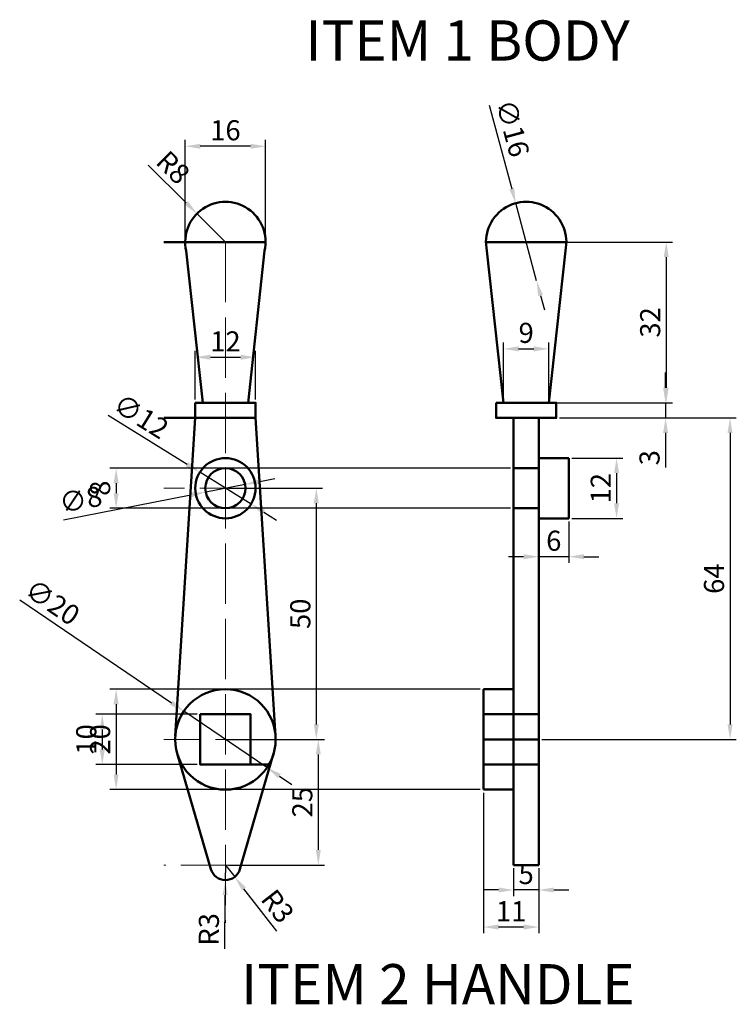
# Model space of a CAD drawing. Units: millimetres. Extents: x 867 to 1199, y -58 to 305.
# Tile 1 of 3: x 906 to 1048, y -58 to 138. Entities that reach past the tile are written whole.
import ezdxf

# ---------------------------------------------------------------- set-up
doc = ezdxf.new("R2010")
doc.units = ezdxf.units.MM
doc.linetypes.add('ACAD_ISO02W100', pattern=[15, 12, -3])
for name, color, linetype, lineweight in [('M-CNTR', 1, 'ACAD_ISO02W100', 18), ('M-DIMS', 2, 'Continuous', 25), ('M-OUTL', 7, 'Continuous', 50), ('M-TEXT', 3, 'Continuous', 25)]:
    doc.layers.add(name, color=color, linetype=linetype, lineweight=lineweight)
doc.styles.get("Standard").update_dxf_attribs({"font": 'arial.ttf'})
doc.dimstyles.new('ISO-25', dxfattribs={"dimtxt": 4, "dimasz": 3, "dimexe": 1.25, "dimexo": 0.625, "dimtad": 1, "dimdec": 1, "dimtxsty": 'Standard', "dimcen": 2.5, "dimadec": 0, "dimazin": 0, "dimtfac": 1, "dimtdec": 1, "dimtmove": 0, "dimatfit": 3, "dimfxl": 1, "dimarcsym": 0})

# ---------------------------------------------------------------- blocks, each defined once
blk = doc.blocks.new('*D18')
at = {"layer": 'Defpoints', "color": 0, "transparency": 16777216}
for p in [(1006.5, 93.39), (1006.5, 61.39), (1034.38, 61.39)]:
    blk.add_point(p, dxfattribs=at)
at = {"layer": 'M-DIMS', "color": 0, "lineweight": -2, "transparency": 16777216}
for p, q in [((1007.12, 93.39), (1035.63, 93.39)), ((1034.38, 90.39), (1034.38, 64.39)), ((1007.12, 61.39), (1035.63, 61.39))]:
    blk.add_line(p, q, dxfattribs=at)
at = {"layer": 'M-DIMS', "color": 0, "transparency": 16777216}
for points in [[(1033.88, 90.39), (1034.88, 90.39), (1034.38, 93.39)], [(1033.88, 64.39), (1034.88, 64.39), (1034.38, 61.39)]]:
    blk.add_solid(points, dxfattribs=at)
at = {"layer": 'M-DIMS', "color": 0, "transparency": 16777216, "insert": (1031.71, 77.39), "char_height": 4, "attachment_point": 5, "rotation": 90}
blk.add_mtext('32', dxfattribs=at)
blk = doc.blocks.new('*D19')
at = {"layer": 'Defpoints', "color": 0, "transparency": 16777216}
for p in [(1012.5, 61.39), (1012.5, 58.39), (1034.25, 58.39)]:
    blk.add_point(p, dxfattribs=at)
at = {"layer": 'M-DIMS', "color": 0, "lineweight": -2, "transparency": 16777216}
for p, q in [((1034.25, 64.39), (1034.25, 67.39)), ((1013.12, 61.39), (1035.5, 61.39)), ((1034.25, 61.39), (1034.25, 58.39)), ((1013.12, 58.39), (1035.5, 58.39)), ((1034.25, 55.39), (1034.25, 48.52))]:
    blk.add_line(p, q, dxfattribs=at)
at = {"layer": 'M-DIMS', "color": 0, "transparency": 16777216}
for points in [[(1033.75, 64.39), (1034.75, 64.39), (1034.25, 61.39)], [(1033.75, 55.39), (1034.75, 55.39), (1034.25, 58.39)]]:
    blk.add_solid(points, dxfattribs=at)
at = {"layer": 'M-DIMS', "color": 0, "transparency": 16777216, "insert": (1031.58, 50.46), "char_height": 4, "attachment_point": 5, "rotation": 90}
blk.add_mtext('3', dxfattribs=at)
blk = doc.blocks.new('*D20')
at = {"layer": 'Defpoints', "color": 0, "transparency": 16777216}
for p in [(1027.13, 58.39), (1009, -5.61), (1047.09, -5.61)]:
    blk.add_point(p, dxfattribs=at)
at = {"layer": 'M-DIMS', "color": 0, "lineweight": -2, "transparency": 16777216}
for p, q in [((1027.76, 58.39), (1048.34, 58.39)), ((1047.09, 55.39), (1047.09, -2.61)), ((1009.62, -5.61), (1048.34, -5.61))]:
    blk.add_line(p, q, dxfattribs=at)
at = {"layer": 'M-DIMS', "color": 0, "transparency": 16777216}
for points in [[(1046.59, 55.39), (1047.59, 55.39), (1047.09, 58.39)], [(1046.59, -2.61), (1047.59, -2.61), (1047.09, -5.61)]]:
    blk.add_solid(points, dxfattribs=at)
at = {"layer": 'M-DIMS', "color": 0, "transparency": 16777216, "insert": (1044.42, 26.39), "char_height": 4, "attachment_point": 5, "rotation": 90}
blk.add_mtext('64', dxfattribs=at)
blk = doc.blocks.new('*D21')
at = {"layer": 'Defpoints', "color": 0, "transparency": 16777216}
for p in [(1009, 38.39), (1015, 38.39), (1009, 30.76)]:
    blk.add_point(p, dxfattribs=at)
at = {"layer": 'M-DIMS', "color": 0, "lineweight": -2, "transparency": 16777216}
for p, q in [((1009, 37.77), (1009, 29.51)), ((1015, 37.77), (1015, 29.51)), ((1006, 30.76), (1003, 30.76)), ((1015, 30.76), (1009, 30.76)), ((1018, 30.76), (1021, 30.76))]:
    blk.add_line(p, q, dxfattribs=at)
at = {"layer": 'M-DIMS', "color": 0, "transparency": 16777216}
for points in [[(1006, 31.26), (1006, 30.26), (1009, 30.76)], [(1018, 31.26), (1018, 30.26), (1015, 30.76)]]:
    blk.add_solid(points, dxfattribs=at)
at = {"layer": 'M-DIMS', "color": 0, "transparency": 16777216, "insert": (1012, 33.42), "char_height": 4, "attachment_point": 5}
blk.add_mtext('6', dxfattribs=at)
blk = doc.blocks.new('*D22')
at = {"layer": 'Defpoints', "color": 0, "transparency": 16777216}
for p in [(1011, 72.13), (1002, 61.39), (1011, 61.39)]:
    blk.add_point(p, dxfattribs=at)
at = {"layer": 'M-DIMS', "color": 0, "lineweight": -2, "transparency": 16777216}
for p, q in [((1002, 62.02), (1002, 73.38)), ((1011, 62.02), (1011, 73.38)), ((1005, 72.13), (1008, 72.13))]:
    blk.add_line(p, q, dxfattribs=at)
at = {"layer": 'M-DIMS', "color": 0, "transparency": 16777216}
for points in [[(1005, 72.63), (1005, 71.63), (1002, 72.13)], [(1008, 72.63), (1008, 71.63), (1011, 72.13)]]:
    blk.add_solid(points, dxfattribs=at)
at = {"layer": 'M-DIMS', "color": 0, "transparency": 16777216, "insert": (1006.5, 74.79), "char_height": 4, "attachment_point": 5}
blk.add_mtext('9', dxfattribs=at)
blk = doc.blocks.new('*D23')
at = {"layer": 'Defpoints', "color": 0, "transparency": 16777216}
for p in [(1004, -30.61), (1009, -30.61), (1004, -35.58)]:
    blk.add_point(p, dxfattribs=at)
at = {"layer": 'M-DIMS', "color": 0, "lineweight": -2, "transparency": 16777216}
for p, q in [((1004, -31.23), (1004, -36.83)), ((1009, -31.23), (1009, -36.83)), ((1001, -35.58), (998, -35.58)), ((1009, -35.58), (1004, -35.58)), ((1012, -35.58), (1015, -35.58))]:
    blk.add_line(p, q, dxfattribs=at)
at = {"layer": 'M-DIMS', "color": 0, "transparency": 16777216}
for points in [[(1001, -35.08), (1001, -36.08), (1004, -35.58)], [(1012, -35.08), (1012, -36.08), (1009, -35.58)]]:
    blk.add_solid(points, dxfattribs=at)
at = {"layer": 'M-DIMS', "color": 0, "transparency": 16777216, "insert": (1006.5, -32.92), "char_height": 4, "attachment_point": 5}
blk.add_mtext('5', dxfattribs=at)
blk = doc.blocks.new('*D24')
at = {"layer": 'Defpoints', "color": 0, "transparency": 16777216}
for p in [(998, -15.61), (1009, -30.61), (998, -42.95)]:
    blk.add_point(p, dxfattribs=at)
at = {"layer": 'M-DIMS', "color": 0, "lineweight": -2, "transparency": 16777216}
for p, q in [((998, -16.23), (998, -44.2)), ((1009, -31.23), (1009, -44.2)), ((1006, -42.95), (1001, -42.95))]:
    blk.add_line(p, q, dxfattribs=at)
at = {"layer": 'M-DIMS', "color": 0, "transparency": 16777216}
for points in [[(1001, -42.45), (1001, -43.45), (998, -42.95)], [(1006, -42.45), (1006, -43.45), (1009, -42.95)]]:
    blk.add_solid(points, dxfattribs=at)
at = {"layer": 'M-DIMS', "color": 0, "transparency": 16777216, "insert": (1003.5, -40.32), "char_height": 4, "attachment_point": 5}
blk.add_mtext('11', dxfattribs=at)
blk = doc.blocks.new('*D25')
at = {"layer": 'Defpoints', "color": 0, "transparency": 16777216}
for p in [(946.63, -5.61), (946.63, -30.61), (965.12, -30.61)]:
    blk.add_point(p, dxfattribs=at)
at = {"layer": 'M-DIMS', "color": 0, "lineweight": -2, "transparency": 16777216}
for p, q in [((947.25, -5.61), (966.37, -5.61)), ((965.12, -8.61), (965.12, -27.61)), ((947.25, -30.61), (966.37, -30.61))]:
    blk.add_line(p, q, dxfattribs=at)
at = {"layer": 'M-DIMS', "color": 0, "transparency": 16777216}
for points in [[(964.62, -8.61), (965.62, -8.61), (965.12, -5.61)], [(964.62, -27.61), (965.62, -27.61), (965.12, -30.61)]]:
    blk.add_solid(points, dxfattribs=at)
at = {"layer": 'M-DIMS', "color": 0, "transparency": 16777216, "insert": (962.45, -18.11), "char_height": 4, "attachment_point": 5, "rotation": 90}
blk.add_mtext('25', dxfattribs=at)
blk = doc.blocks.new('*D26')
at = {"layer": 'Defpoints', "color": 0, "transparency": 16777216}
for p in [(946.63, 44.39), (946.63, -5.61), (964.72, -5.61)]:
    blk.add_point(p, dxfattribs=at)
at = {"layer": 'M-DIMS', "color": 0, "lineweight": -2, "transparency": 16777216}
for p, q in [((947.25, 44.39), (965.97, 44.39)), ((964.72, 41.39), (964.72, -2.61)), ((947.25, -5.61), (965.97, -5.61))]:
    blk.add_line(p, q, dxfattribs=at)
at = {"layer": 'M-DIMS', "color": 0, "transparency": 16777216}
for points in [[(964.22, 41.39), (965.22, 41.39), (964.72, 44.39)], [(964.22, -2.61), (965.22, -2.61), (964.72, -5.61)]]:
    blk.add_solid(points, dxfattribs=at)
at = {"layer": 'M-DIMS', "color": 0, "transparency": 16777216, "insert": (962.05, 19.39), "char_height": 4, "attachment_point": 5, "rotation": 90}
blk.add_mtext('50', dxfattribs=at)
blk = doc.blocks.new('*D27')
at = {"layer": 'Defpoints', "color": 0, "transparency": 16777216}
for p in [(952.63, 70.46), (940.63, 61.39), (952.63, 61.39)]:
    blk.add_point(p, dxfattribs=at)
at = {"layer": 'M-DIMS', "color": 0, "lineweight": -2, "transparency": 16777216}
for p, q in [((940.63, 62.02), (940.63, 71.71)), ((952.63, 62.02), (952.63, 71.71)), ((943.63, 70.46), (949.63, 70.46))]:
    blk.add_line(p, q, dxfattribs=at)
at = {"layer": 'M-DIMS', "color": 0, "transparency": 16777216}
for points in [[(943.63, 70.96), (943.63, 69.96), (940.63, 70.46)], [(949.63, 70.96), (949.63, 69.96), (952.63, 70.46)]]:
    blk.add_solid(points, dxfattribs=at)
at = {"layer": 'M-DIMS', "color": 0, "transparency": 16777216, "insert": (946.63, 73.09), "char_height": 4, "attachment_point": 5}
blk.add_mtext('12', dxfattribs=at)
blk = doc.blocks.new('*D28')
at = {"layer": 'Defpoints', "color": 0, "transparency": 16777216}
for p in [(938.63, 112.45), (938.63, 93.39), (954.63, 93.39)]:
    blk.add_point(p, dxfattribs=at)
at = {"layer": 'M-DIMS', "color": 0, "lineweight": -2, "transparency": 16777216}
for p, q in [((938.63, 94.02), (938.63, 113.7)), ((954.63, 94.02), (954.63, 113.7)), ((951.63, 112.45), (941.63, 112.45))]:
    blk.add_line(p, q, dxfattribs=at)
at = {"layer": 'M-DIMS', "color": 0, "transparency": 16777216}
for points in [[(941.63, 112.95), (941.63, 111.95), (938.63, 112.45)], [(951.63, 112.95), (951.63, 111.95), (954.63, 112.45)]]:
    blk.add_solid(points, dxfattribs=at)
at = {"layer": 'M-DIMS', "color": 0, "transparency": 16777216, "insert": (946.63, 115.12), "char_height": 4, "attachment_point": 5}
blk.add_mtext('16', dxfattribs=at)
blk = doc.blocks.new('*D29')
at = {"layer": 'Defpoints', "color": 0, "transparency": 16777216}
for p in [(1004.42, 101.12), (1008.58, 85.67)]:
    blk.add_point(p, dxfattribs=at)
at = {"layer": 'M-DIMS', "color": 0, "lineweight": -2, "transparency": 16777216}
for p, q in [((999.16, 120.64), (1003.64, 104.01)), ((1008.58, 85.67), (1004.42, 101.12)), ((1009.36, 82.77), (1010.14, 79.88))]:
    blk.add_line(p, q, dxfattribs=at)
at = {"layer": 'M-DIMS', "color": 0, "transparency": 16777216}
for points in [[(1004.12, 104.14), (1003.15, 103.88), (1004.42, 101.12)], [(1009.84, 82.9), (1008.88, 82.64), (1008.58, 85.67)]]:
    blk.add_solid(points, dxfattribs=at)
at = {"layer": 'M-DIMS', "color": 0, "transparency": 16777216, "insert": (1003.31, 115.9), "char_height": 4, "attachment_point": 5, "rotation": 285.0798}
blk.add_mtext('∅16', dxfattribs=at)
blk = doc.blocks.new('*D30')
at = {"layer": 'Defpoints', "color": 0, "transparency": 16777216}
for p in [(938.35, 0), (954.9, -11.22)]:
    blk.add_point(p, dxfattribs=at)
at = {"layer": 'M-DIMS', "color": 0, "lineweight": -2, "transparency": 16777216}
for p, q in [((905.67, 22.16), (935.87, 1.69)), ((954.9, -11.22), (938.35, 0)), ((957.39, -12.9), (959.87, -14.58))]:
    blk.add_line(p, q, dxfattribs=at)
at = {"layer": 'M-DIMS', "color": 0, "transparency": 16777216}
for points in [[(936.15, 2.1), (935.59, 1.27), (938.35, 0)], [(957.67, -12.49), (957.11, -13.31), (954.9, -11.22)]]:
    blk.add_solid(points, dxfattribs=at)
at = {"layer": 'M-DIMS', "color": 0, "transparency": 16777216, "insert": (911.91, 21.28), "char_height": 4, "attachment_point": 5, "rotation": 325.8689}
blk.add_mtext('∅20', dxfattribs=at)
blk = doc.blocks.new('*D31')
at = {"layer": 'Defpoints', "color": 0, "transparency": 16777216}
for p in [(941.53, 47.56), (951.72, 41.23)]:
    blk.add_point(p, dxfattribs=at)
at = {"layer": 'M-DIMS', "color": 0, "lineweight": -2, "transparency": 16777216}
for p, q in [((923.3, 58.9), (938.98, 49.15)), ((951.72, 41.23), (941.53, 47.56)), ((954.27, 39.64), (956.82, 38.06))]:
    blk.add_line(p, q, dxfattribs=at)
at = {"layer": 'M-DIMS', "color": 0, "transparency": 16777216}
for points in [[(939.25, 49.57), (938.72, 48.72), (941.53, 47.56)], [(954.53, 40.07), (954.01, 39.22), (951.72, 41.23)]]:
    blk.add_solid(points, dxfattribs=at)
at = {"layer": 'M-DIMS', "color": 0, "transparency": 16777216, "insert": (929.56, 58.28), "char_height": 4, "attachment_point": 5, "rotation": 328.1301}
blk.add_mtext('∅12', dxfattribs=at)
blk = doc.blocks.new('*D32')
at = {"layer": 'Defpoints', "color": 0, "transparency": 16777216}
for p in [(950.55, 45.16), (942.7, 43.63)]:
    blk.add_point(p, dxfattribs=at)
at = {"layer": 'M-DIMS', "color": 0, "lineweight": -2, "transparency": 16777216}
for p, q in [((950.55, 45.16), (942.7, 43.63)), ((953.5, 45.73), (956.44, 46.31)), ((914.39, 38.12), (939.76, 43.06))]:
    blk.add_line(p, q, dxfattribs=at)
at = {"layer": 'M-DIMS', "color": 0, "transparency": 16777216}
for points in [[(953.4, 46.22), (953.59, 45.24), (950.55, 45.16)], [(939.66, 43.55), (939.85, 42.56), (942.7, 43.63)]]:
    blk.add_solid(points, dxfattribs=at)
at = {"layer": 'M-DIMS', "color": 0, "transparency": 16777216, "insert": (917.9, 41.63), "char_height": 4, "attachment_point": 5, "rotation": 11.0212}
blk.add_mtext('∅8', dxfattribs=at)
blk = doc.blocks.new('*D33')
at = {"layer": 'Defpoints', "color": 0, "transparency": 16777216}
for p in [(946.63, -30.61), (948.47, -32.98)]:
    blk.add_point(p, dxfattribs=at)
at = {"layer": 'M-DIMS', "color": 0, "lineweight": -2, "transparency": 16777216}
for p, q in [((946.63, -30.61), (948.47, -32.98)), ((956.87, -43.8), (950.31, -35.35))]:
    blk.add_line(p, q, dxfattribs=at)
at = {"layer": 'M-DIMS', "color": 0, "transparency": 16777216}
blk.add_solid([(950.7, -35.04), (949.91, -35.65), (948.47, -32.98)], dxfattribs=at)
at = {"layer": 'M-DIMS', "color": 0, "transparency": 16777216, "insert": (956.62, -39.12), "char_height": 4, "attachment_point": 5, "rotation": 307.8372}
blk.add_mtext('R3', dxfattribs=at)
blk = doc.blocks.new('*D34')
at = {"layer": 'Defpoints', "color": 0, "transparency": 16777216}
for p in [(941.63, -0.61), (922.11, -10.61), (941.63, -10.61)]:
    blk.add_point(p, dxfattribs=at)
at = {"layer": 'M-DIMS', "color": 0, "lineweight": -2, "transparency": 16777216}
for p, q in [((941, -0.61), (920.86, -0.61)), ((922.11, -3.61), (922.11, -7.61)), ((941, -10.61), (920.86, -10.61))]:
    blk.add_line(p, q, dxfattribs=at)
at = {"layer": 'M-DIMS', "color": 0, "transparency": 16777216}
for points in [[(921.61, -3.61), (922.61, -3.61), (922.11, -0.61)], [(921.61, -7.61), (922.61, -7.61), (922.11, -10.61)]]:
    blk.add_solid(points, dxfattribs=at)
at = {"layer": 'M-DIMS', "color": 0, "transparency": 16777216, "insert": (919.44, -5.61), "char_height": 4, "attachment_point": 5, "rotation": 90}
blk.add_mtext('10', dxfattribs=at)
blk = doc.blocks.new('*D57')
at = {"layer": 'Defpoints', "color": 0, "transparency": 16777216}
for p in [(998, 4.39), (924.87, -15.61), (998, -15.61)]:
    blk.add_point(p, dxfattribs=at)
at = {"layer": 'M-DIMS', "color": 0, "lineweight": -2, "transparency": 16777216}
for p, q in [((997.37, 4.39), (923.62, 4.39)), ((924.87, 1.39), (924.87, -12.61)), ((997.37, -15.61), (923.62, -15.61))]:
    blk.add_line(p, q, dxfattribs=at)
at = {"layer": 'M-DIMS', "color": 0, "transparency": 16777216}
for points in [[(924.37, 1.39), (925.37, 1.39), (924.87, 4.39)], [(924.37, -12.61), (925.37, -12.61), (924.87, -15.61)]]:
    blk.add_solid(points, dxfattribs=at)
at = {"layer": 'M-DIMS', "color": 0, "transparency": 16777216, "insert": (922.2, -5.61), "char_height": 4, "attachment_point": 5, "rotation": 90}
blk.add_mtext('20', dxfattribs=at)
blk = doc.blocks.new('*D58')
at = {"layer": 'Defpoints', "color": 0, "transparency": 16777216}
for p in [(1015, 50.39), (1015, 38.39), (1024.5, 38.39)]:
    blk.add_point(p, dxfattribs=at)
at = {"layer": 'M-DIMS', "color": 0, "lineweight": -2, "transparency": 16777216}
for p, q in [((1015.62, 50.39), (1025.75, 50.39)), ((1024.5, 47.39), (1024.5, 41.39)), ((1015.62, 38.39), (1025.75, 38.39))]:
    blk.add_line(p, q, dxfattribs=at)
at = {"layer": 'M-DIMS', "color": 0, "transparency": 16777216}
for points in [[(1024, 47.39), (1025, 47.39), (1024.5, 50.39)], [(1024, 41.39), (1025, 41.39), (1024.5, 38.39)]]:
    blk.add_solid(points, dxfattribs=at)
at = {"layer": 'M-DIMS', "color": 0, "transparency": 16777216, "insert": (1021.87, 44.39), "char_height": 4, "attachment_point": 5, "rotation": 90}
blk.add_mtext('12', dxfattribs=at)
blk = doc.blocks.new('*D59')
at = {"layer": 'Defpoints', "color": 0, "transparency": 16777216}
for p in [(1004, 48.39), (924.87, 40.39), (1004, 40.39)]:
    blk.add_point(p, dxfattribs=at)
at = {"layer": 'M-DIMS', "color": 0, "lineweight": -2, "transparency": 16777216}
for p, q in [((1003.37, 48.39), (923.62, 48.39)), ((924.87, 45.39), (924.87, 43.39)), ((1003.37, 40.39), (923.62, 40.39))]:
    blk.add_line(p, q, dxfattribs=at)
at = {"layer": 'M-DIMS', "color": 0, "transparency": 16777216}
for points in [[(924.37, 45.39), (925.37, 45.39), (924.87, 48.39)], [(924.37, 43.39), (925.37, 43.39), (924.87, 40.39)]]:
    blk.add_solid(points, dxfattribs=at)
at = {"layer": 'M-DIMS', "color": 0, "transparency": 16777216, "insert": (922.2, 44.39), "char_height": 4, "attachment_point": 5, "rotation": 90}
blk.add_mtext('8', dxfattribs=at)
blk = doc.blocks.new('*D65')
at = {"layer": 'Defpoints', "color": 0, "transparency": 16777216}
for p in [(946.63, -30.61), (946.6, -33.61)]:
    blk.add_point(p, dxfattribs=at)
at = {"layer": 'M-DIMS', "color": 0, "lineweight": -2, "transparency": 16777216}
for p, q in [((946.63, -30.61), (946.6, -33.61)), ((946.48, -47.31), (946.57, -36.61))]:
    blk.add_line(p, q, dxfattribs=at)
at = {"layer": 'M-DIMS', "color": 0, "transparency": 16777216}
blk.add_solid([(946.07, -36.6), (947.07, -36.61), (946.6, -33.61)], dxfattribs=at)
at = {"layer": 'M-DIMS', "color": 0, "transparency": 16777216, "insert": (943.84, -43.43), "char_height": 4, "attachment_point": 5, "rotation": 89.4844}
blk.add_mtext('R3', dxfattribs=at)
blk = doc.blocks.new('*D66')
at = {"layer": 'Defpoints', "color": 0, "transparency": 16777216}
for p in [(940.96, 99.04), (946.63, 93.39)]:
    blk.add_point(p, dxfattribs=at)
at = {"layer": 'M-DIMS', "color": 0, "lineweight": -2, "transparency": 16777216}
for p, q in [((931.25, 108.72), (938.83, 101.16)), ((946.63, 93.39), (940.96, 99.04))]:
    blk.add_line(p, q, dxfattribs=at)
at = {"layer": 'M-DIMS', "color": 0, "transparency": 16777216}
blk.add_solid([(939.19, 101.51), (938.48, 100.8), (940.96, 99.04)], dxfattribs=at)
at = {"layer": 'M-DIMS', "color": 0, "transparency": 16777216, "insert": (935.86, 107.88), "char_height": 4, "attachment_point": 5, "rotation": 315.104}
blk.add_mtext('R8', dxfattribs=at)

msp = doc.modelspace()

# ---------------------------------------------------------------- linework, layer by layer
at = {"layer": 'M-CNTR'}
for p, q in [((946.627, 93.393), (946.627, -42.094)), ((953.506, 44.393), (934.366, 44.393)), ((956.627, -5.607), (934.366, -5.607)), ((949.752, -30.607), (934.366, -30.607))]:
    msp.add_line(p, q, dxfattribs=at)
at = {"layer": 'M-OUTL'}
for p, q in [((954.627, 93.393), (934.366, 93.393)), ((1014.5, 93.393), (998.5, 93.393)), ((952.627, 58.393), (934.366, 58.393)), ((940.627, 58.393), (936.647, -4.98)), ((952.627, 58.393), (956.607, -4.98)), ((1012.5, 58.393), (1000.5, 58.393)), ((1004, 58.393), (1004, -30.607)), ((1009, 58.393), (1009, -30.607)), ((1009, 50.393), (1015, 50.393)), ((1015, 38.393), (1015, 50.393)), ((1004, 48.393), (1009, 48.393)), ((1004, 40.393), (1009, 40.393)), ((1009, 38.393), (1015, 38.393)), ((998, 4.393), (998, -15.607)), ((998, 4.393), (1004, 4.393)), ((946.627, -0.607), (951.627, -0.607)), ((998, -0.607), (1009, -0.607)), ((1009, -5.607), (998, -5.607)), ((937.027, -8.407), (943.747, -31.447)), ((956.227, -8.407), (949.507, -31.447)), ((946.627, -10.607), (955.287, -10.607)), ((998, -10.607), (1009, -10.607)), ((998, -15.607), (1004, -15.607)), ((1009, -30.607), (1004, -30.607))]:
    msp.add_line(p, q, dxfattribs=at)
for points in [[(951.127, 61.393), (954.438, 91.664, 1.245614), (938.816, 91.664), (942.127, 61.393)], [(1011, 61.393), (1014.31, 91.664, 1.245614), (998.689, 91.664), (1002, 61.393)]]:
    msp.add_lwpolyline(points, format="xyb", dxfattribs=at)
for points in [[(940.627, 61.393), (952.627, 61.393), (952.627, 58.393), (940.627, 58.393)], [(1000.5, 61.393), (1012.5, 61.393), (1012.5, 58.393), (1000.5, 58.393)], [(941.627, -0.607), (951.627, -0.607), (951.627, -10.607), (941.627, -10.607)]]:
    msp.add_lwpolyline(points, close=True, dxfattribs=at)
for centre, radius in [((946.627, 44.393), 6), ((946.627, 44.393), 4), ((946.627, -5.607), 10)]:
    msp.add_circle(centre, radius, dxfattribs=at)
msp.add_arc((946.627, -30.607), 3, 196.2602, 343.7398, dxfattribs=at)

# ---------------------------------------------------------------- texts
at = {"layer": 'M-TEXT', "char_height": 8, "attachment_point": 1}
for s, insert in [('ITEM 1 BODY', (962.582, 137.503)), ('ITEM 2 HANDLE', (949.773, -50.333))]:
    msp.add_mtext_dynamic_manual_height_columns(s, width=84.35545, gutter_width=12.5, heights=[0], dxfattribs=dict(at, insert=insert))

# ---------------------------------------------------------------- dimensions: what is measured, and where the dimension line sits
at = {"layer": 'M-DIMS'}
for p1, p2, picture, middle in [((1008.581, 85.669), (1004.418, 101.118), '*D29', (1000.631, 115.173)), ((951.722, 41.226), (941.531, 47.561), '*D31', (928.093, 55.917)), ((950.553, 45.158), (942.701, 43.629), '*D32', (918.434, 38.903)), ((954.904, -11.217), (938.349, 0.004), '*D30', (910.352, 18.982))]:
    dim = msp.add_diameter_dim_2p(p1=p1, p2=p2, dimstyle='ISO-25', override={"dimclrd": 0, "dimclre": 0, "dimclrt": 0}, dxfattribs=at)
    dim.commit()
    dim.dimension.update_dxf_attribs({"geometry": picture, "text_midpoint": middle, "dimtype": 163})
for base, p1, p2, picture, middle in [((938.627, 112.449), (954.627, 93.393), (938.627, 93.393), '*D28', (946.627, 115.117)), ((1011, 72.126), (1002, 61.393), (1011, 61.393), '*D22', (1006.5, 74.794)), ((952.627, 70.461), (940.627, 61.393), (952.627, 61.393), '*D27', (946.627, 73.094)), ((1009, 30.758), (1015, 38.393), (1009, 38.393), '*D21', (1012, 33.425)), ((998, -42.95), (1009, -30.607), (998, -15.607), '*D24', (1003.5, -40.316)), ((1004, -35.583), (1009, -30.607), (1004, -30.607), '*D23', (1006.5, -32.923))]:
    dim = msp.add_linear_dim(base=base, p1=p1, p2=p2, dimstyle='ISO-25', override={"dimclrd": 0, "dimclre": 0, "dimclrt": 0}, dxfattribs=at)
    dim.commit()
    dim.dimension.update_dxf_attribs({"geometry": picture, "text_midpoint": middle})
for center, mpoint, override, picture, middle in [((946.627, 93.393), (940.96, 99.04), {"dimdec": 0, "dimlfac": 1, "dimrnd": 0, "dimzin": 0, "dimdsep": 46, "dimlunit": 2}, '*D66', (935.862, 107.885)), ((946.627, -30.607), (946.6, -33.606), {"dimdec": 0, "dimlfac": 1, "dimrnd": 0, "dimzin": 0, "dimdsep": 46, "dimlunit": 2}, '*D65', (943.843, -43.432)), ((946.627, -30.607), (948.467, -32.976), {"dimclrd": 0, "dimclre": 0, "dimclrt": 0}, '*D33', (956.617, -39.118))]:
    dim = msp.add_radius_dim(center=center, mpoint=mpoint, dimstyle='ISO-25', override=override, dxfattribs=at)
    dim.commit()
    dim.dimension.update_dxf_attribs({"geometry": picture, "text_midpoint": middle})
for base, p1, p2, override, picture, middle in [((1034.378, 61.393), (1006.5, 93.393), (1006.5, 61.393), {"dimclrd": 0, "dimclre": 0, "dimclrt": 0}, '*D18', (1031.71, 77.393)), ((1034.247, 58.393), (1012.5, 61.393), (1012.5, 58.393), {"dimclrd": 0, "dimclre": 0, "dimclrt": 0}, '*D19', (1031.578, 50.459)), ((1047.088, -5.607), (1027.135, 58.393), (1009, -5.607), {"dimclrd": 0, "dimclre": 0, "dimclrt": 0}, '*D20', (1044.42, 26.393)), ((1024.5, 38.393), (1015, 50.393), (1015, 38.393), {"dimdec": 0, "dimlfac": 1, "dimrnd": 0, "dimzin": 0, "dimdsep": 46, "dimlunit": 2}, '*D58', (1021.866, 44.393)), ((924.866, 40.393), (1004, 48.393), (1004, 40.393), {"dimdec": 0, "dimlfac": 1, "dimrnd": 0, "dimzin": 0, "dimdsep": 46, "dimlunit": 2}, '*D59', (922.199, 44.393)), ((964.719, -5.607), (946.627, 44.393), (946.627, -5.607), {"dimclrd": 0, "dimclre": 0, "dimclrt": 0}, '*D26', (962.052, 19.393)), ((924.866, -15.607), (998, 4.393), (998, -15.607), {"dimdec": 0, "dimlfac": 1, "dimrnd": 0, "dimzin": 0, "dimdsep": 46, "dimlunit": 2}, '*D57', (922.199, -5.607)), ((922.108, -10.607), (941.627, -0.607), (941.627, -10.607), {"dimclrd": 0, "dimclre": 0, "dimclrt": 0}, '*D34', (919.44, -5.607)), ((965.116, -30.607), (946.627, -5.607), (946.627, -30.607), {"dimclrd": 0, "dimclre": 0, "dimclrt": 0}, '*D25', (962.448, -18.107))]:
    dim = msp.add_linear_dim(base=base, p1=p1, p2=p2, angle=90, dimstyle='ISO-25', override=override, dxfattribs=at)
    dim.commit()
    dim.dimension.update_dxf_attribs({"geometry": picture, "text_midpoint": middle})

doc.saveas('drawing.dxf')
